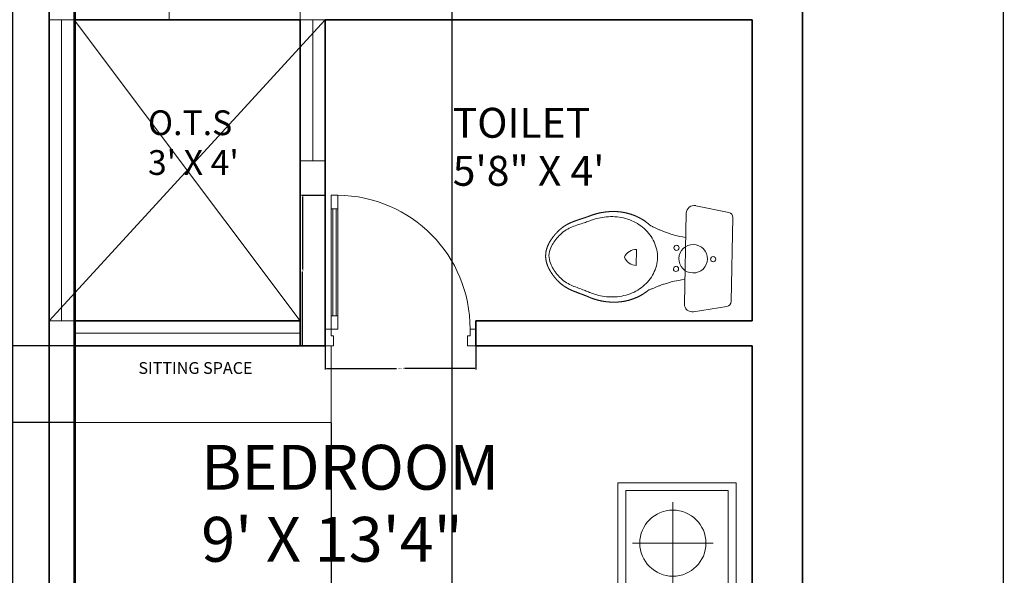
# Model space of a CAD drawing. Units: feet. Extents: x 1993 to 2298, y 2938 to 3641.
# Tile 10 of 11: x 2141 to 2298, y 3468 to 3557. Entities that reach past the tile are written whole.
import ezdxf

# ---------------------------------------------------------------- set-up
doc = ezdxf.new("R2010")
doc.units = ezdxf.units.FT
for name, color, linetype, lineweight in [('A-ANNO-DIMS', 2, 'Continuous', 18), ('A-AREA-IDEN', 7, 'Continuous', 18), ('A-DOOR', 3, 'Continuous', 18), ('A-FLOR-CASE', 8, 'Continuous', 18), ('A-FLOR-FIXT', 9, 'Continuous', 18), ('A-FLOR-OPEN', 8, 'Continuous', 13), ('A-GLAZ', 4, 'Continuous', 13), ('DWV_RED', 7, 'Continuous', 0), ('furniture', 8, 'Continuous', 18), ('WAL', 7, 'Continuous', 35)]:
    doc.layers.add(name, color=color, linetype=linetype, lineweight=lineweight)
doc.styles.add('DIM_FONT', font='SIMPLEX.shx', dxfattribs={"width": 0.8})
doc.styles.get("Standard").update_dxf_attribs({"font": 'arial.ttf'})
doc.dimstyles.get("Standard").update_dxf_attribs({"dimtxt": 0.18, "dimasz": 0.18, "dimexe": 0.18, "dimexo": 0.0625, "dimgap": 0.09, "dimtad": 0, "dimtih": 1, "dimtoh": 1, "dimdec": 4, "dimzin": 0, "dimdsep": 46, "dimtxsty": 'Standard', "dimcen": 0.09, "dimadec": 0, "dimazin": 0, "dimtfac": 1, "dimtdec": 4, "dimtofl": 0, "dimtmove": 0, "dimatfit": 3, "dimfxl": 1, "dimtolj": 1, "dimtzin": 0, "dimarcsym": 0})

# ---------------------------------------------------------------- blocks, each defined once
blk = doc.blocks.new('A$C184E58E8')
for points in [[(825, 900), (825, 820), (865, 820), (865, 900)], [(825, 180), (825, 820), (865, 820), (865, 180)], [(835, 180), (835, 820), (855, 820), (855, 180)], [(825, 100), (825, 180), (865, 180), (865, 100)], [(35, 100), (35, 60), (50, 60), (50, 50), (50, 0), (0, 0), (0, 100)], [(865, 100), (900, 100), (900, 0), (850, 0), (850, 50), (850, 60), (865, 60)]]:
    blk.add_lwpolyline(points, close=True)
blk.add_arc((830, 105), 795, 90.36035, 180.36035)
blk = doc.blocks.new('A$C79766A75')
for p, q in [((0.45, 1.9999), (0, 1.9999)), ((0, 1.9999), (0, 1.5499)), ((0.42, 1.9699), (0.03, 1.9699)), ((0.03, 1.9699), (0.03, 1.5799)), ((0.2304, 1.9125), (0.2304, 1.6061)), ((0.0743, 1.7595), (0.3834, 1.7595)), ((0.03, 1.5799), (0.42, 1.5799)), ((0, 1.5499), (0.45, 1.5499))]:
    blk.add_line(p, q)
blk.add_circle((0.2304, 1.7595), 0.126)
at = {"style": 'DIM_FONT', "text_generation_flag": 4, "width": 0.8, "flags": 9}
for tag in ['XSIZE', 'YSIZE']:
    blk.add_attdef(tag, (1.9506, 2), '', height=0.0005, rotation=180, dxfattribs=at)
blk = doc.blocks.new('A$C6F4D5F33')
at = {"layer": 'DWV_RED'}
for p, q in [((142.3, 403.6), (16.1, 380.5)), ((177.2, 29.5), (177.2, 374.6)), ((0, 42.9), (0, 361.2)), ((376.2, 337), (368.9, 333.5)), ((383.7, 340.2), (376.2, 337)), ((391.3, 343.1), (383.7, 340.2)), ((399.1, 345.6), (391.3, 343.1)), ((407, 347.8), (399.1, 345.6)), ((415, 349.7), (407, 347.8)), ((423.1, 351.2), (415, 349.7)), ((431.3, 352.5), (423.1, 351.2)), ((439.5, 353.3), (431.3, 352.5)), ((447.9, 353.8), (439.5, 353.3)), ((456.2, 354), (447.9, 353.8)), ((464.5, 353.9), (456.2, 354)), ((472.6, 353.4), (464.5, 353.9)), ((480.5, 352.6), (472.6, 353.4)), ((488.1, 351.6), (480.5, 352.6)), ((495.5, 350.4), (488.1, 351.6)), ((502.6, 349.1), (495.5, 350.4)), ((509.4, 347.5), (502.6, 349.1)), ((515.8, 345.9), (509.4, 347.5)), ((521.9, 344.1), (515.8, 345.9)), ((527.5, 342.3), (521.9, 344.1)), ((532.7, 340.4), (527.5, 342.3)), ((537.5, 338.6), (532.7, 340.4)), ((542, 336.9), (537.5, 338.6)), ((546.2, 335.2), (542, 336.9)), ((324, 300.1), (318.7, 294.3)), ((329.7, 305.8), (324, 300.1)), ((335.6, 311.2), (329.7, 305.8)), ((341.8, 316.3), (335.6, 311.2)), ((348.2, 321), (341.8, 316.3)), ((354.9, 325.5), (348.2, 321)), ((361.8, 329.7), (354.9, 325.5)), ((368.9, 333.5), (361.8, 329.7)), ((550.3, 333.5), (546.2, 335.2)), ((554.5, 331.9), (550.3, 333.5)), ((558.9, 330.3), (554.5, 331.9)), ((563.7, 328.6), (558.9, 330.3)), ((568.9, 326.8), (563.7, 328.6)), ((574.3, 324.9), (568.9, 326.8)), ((579.9, 323), (574.3, 324.9)), ((585.7, 321), (579.9, 323)), ((591.4, 318.9), (585.7, 321)), ((597.2, 316.8), (591.4, 318.9)), ((602.9, 314.5), (597.2, 316.8)), ((608.6, 312.1), (602.9, 314.5)), ((614.3, 309.5), (608.6, 312.1)), ((620, 306.6), (614.3, 309.5)), ((625.7, 303.4), (620, 306.6)), ((631.4, 299.9), (625.7, 303.4)), ((637, 296.1), (631.4, 299.9)), ((300.6, 268.4), (296.9, 261.5)), ((304.6, 275.2), (300.6, 268.4)), ((309, 281.8), (304.6, 275.2)), ((313.7, 288.1), (309, 281.8)), ((318.7, 294.3), (313.7, 288.1)), ((642.4, 291.8), (637, 296.1)), ((647.7, 287.3), (642.4, 291.8)), ((652.6, 282.7), (647.7, 287.3)), ((657.3, 277.9), (652.6, 282.7)), ((661.7, 273), (657.3, 277.9)), ((665.8, 268), (661.7, 273)), ((669.7, 263), (665.8, 268)), ((673.4, 258), (669.7, 263)), ((284.8, 224.5), (283.7, 216.9)), ((286.4, 232.1), (284.8, 224.5)), ((288.4, 239.6), (286.4, 232.1)), ((290.8, 247), (288.4, 239.6)), ((293.7, 254.3), (290.8, 247)), ((296.9, 261.5), (293.7, 254.3)), ((362.6, 232.5), (362.6, 171.6)), ((676.8, 253), (673.4, 258)), ((680.1, 247.8), (676.8, 253)), ((683.2, 242.5), (680.1, 247.8)), ((686.1, 236.7), (683.2, 242.5)), ((688.7, 230.6), (686.1, 236.7)), ((691.1, 224), (688.7, 230.6)), ((283.1, 209.2), (282.8, 201.5)), ((282.8, 201.5), (283.1, 193.8)), ((283.7, 216.9), (283.1, 209.2)), ((283.1, 193.8), (283.7, 186.1)), ((692.9, 217), (691.1, 224)), ((694.1, 209.4), (692.9, 217)), ((692.9, 186.1), (694.1, 193.6)), ((694.6, 201.5), (694.1, 209.4)), ((694.1, 193.6), (694.6, 201.5)), ((283.7, 186.1), (284.8, 178.4)), ((284.8, 178.4), (286.4, 170.8)), ((286.4, 170.8), (288.4, 163.3)), ((288.4, 163.3), (290.8, 155.9)), ((290.8, 155.9), (293.7, 148.6)), ((673.4, 145), (676.8, 150.1)), ((676.8, 150.1), (680.1, 155.2)), ((680.1, 155.2), (683.2, 160.6)), ((683.2, 160.6), (686.1, 166.3)), ((686.1, 166.3), (688.7, 172.4)), ((688.7, 172.4), (691.1, 179)), ((691.1, 179), (692.9, 186.1)), ((293.7, 148.6), (296.9, 141.5)), ((296.9, 141.5), (300.6, 134.5)), ((300.6, 134.5), (304.6, 127.7)), ((304.6, 127.7), (309, 121.2)), ((309, 121.2), (313.7, 114.8)), ((313.7, 114.8), (318.7, 108.7)), ((642.4, 111.2), (647.7, 115.7)), ((647.7, 115.7), (652.6, 120.4)), ((652.6, 120.4), (657.3, 125.2)), ((657.3, 125.2), (661.7, 130.1)), ((661.7, 130.1), (665.8, 135)), ((665.8, 135), (669.7, 140)), ((669.7, 140), (673.4, 145)), ((318.7, 108.7), (324, 102.8)), ((324, 102.8), (329.7, 97.2)), ((329.7, 97.2), (335.6, 91.8)), ((335.6, 91.8), (341.8, 86.7)), ((341.8, 86.7), (348.2, 81.9)), ((348.2, 81.9), (354.9, 77.4)), ((354.9, 77.4), (361.8, 73.3)), ((564, 74.5), (569.1, 76.3)), ((569.1, 76.3), (574.6, 78.2)), ((574.6, 78.2), (580.1, 80.1)), ((580.1, 80.1), (585.8, 82.1)), ((585.8, 82.1), (591.5, 84.2)), ((591.5, 84.2), (597.2, 86.3)), ((597.2, 86.3), (602.9, 88.6)), ((602.9, 88.6), (608.6, 91)), ((608.6, 91), (614.3, 93.6)), ((614.3, 93.6), (620, 96.4)), ((620, 96.4), (625.7, 99.6)), ((625.7, 99.6), (631.4, 103.1)), ((631.4, 103.1), (637, 107)), ((637, 107), (642.4, 111.2)), ((361.8, 73.3), (368.9, 69.4)), ((368.9, 69.4), (376.2, 65.9)), ((376.2, 65.9), (383.7, 62.7)), ((383.7, 62.7), (391.3, 59.8)), ((391.3, 59.8), (399.1, 57.3)), ((399.1, 57.3), (407, 55.1)), ((407, 55.1), (415, 53.2)), ((415, 53.2), (423.1, 51.7)), ((423.1, 51.7), (431.3, 50.5)), ((431.3, 50.5), (439.5, 49.6)), ((439.5, 49.6), (447.9, 49.1)), ((447.9, 49.1), (456.2, 48.9)), ((456.2, 48.9), (464.5, 49.1)), ((464.5, 49.1), (472.6, 49.6)), ((472.6, 49.6), (480.5, 50.3)), ((480.5, 50.3), (488.1, 51.3)), ((488.1, 51.3), (495.5, 52.5)), ((495.5, 52.5), (502.7, 53.9)), ((502.7, 53.9), (509.5, 55.4)), ((509.5, 55.4), (515.9, 57.1)), ((515.9, 57.1), (522, 58.9)), ((522, 58.9), (527.7, 60.8)), ((527.7, 60.8), (532.9, 62.6)), ((532.9, 62.6), (537.7, 64.5)), ((537.7, 64.5), (542.3, 66.2)), ((542.3, 66.2), (546.5, 68)), ((546.5, 68), (550.6, 69.6)), ((550.6, 69.6), (554.8, 71.2)), ((554.8, 71.2), (559.2, 72.8)), ((559.2, 72.8), (564, 74.5)), ((142.3, 0.5), (16.1, 23.6))]:
    blk.add_line(p, q, dxfattribs=at)
blk.add_lwpolyline([(177.2, 282.1), (189.7, 283.7), (200.3, 285.4), (209.4, 287.1), (217.2, 288.8), (223.8, 290.5), (229.5, 292.2), (234.5, 293.8), (239, 295.3), (243.3, 296.8), (247.4, 298.1), (251.3, 299.4), (254.9, 300.6), (258.4, 301.7), (261.7, 302.9), (264.8, 304), (267.8, 305.1), (270.6, 306.2), (273.3, 307.3), (275.9, 308.4), (278.5, 309.5), (281.1, 310.7), (283.7, 311.9), (286.3, 313.1), (289.1, 314.3), (291.9, 315.5), (294.8, 316.8), (297.7, 318), (300.5, 319.2), (303.3, 320.3), (305.8, 321.4), (308, 322.3), (310, 323.2), (311.5, 323.8), (312.8, 324.4), (313.8, 324.9), (314.6, 325.3), (315.2, 325.7), (315.7, 326), (316.2, 326.4), (316.7, 326.8), (317.3, 327.3), (318, 327.8), (318.7, 328.4), (319.5, 329), (320.3, 329.7), (321.1, 330.3), (322, 331), (322.9, 331.7), (323.8, 332.4), (324.7, 333.1), (325.6, 333.8), (326.5, 334.4), (327.4, 335.1), (328.3, 335.8), (329.2, 336.4), (330.1, 337.1), (331, 337.7), (331.9, 338.3), (332.9, 339), (333.8, 339.6), (334.7, 340.2), (335.7, 340.8), (336.6, 341.5), (337.6, 342.1), (338.5, 342.7), (339.5, 343.3), (340.4, 343.8), (341.4, 344.4), (342.3, 345), (343.3, 345.6), (344.3, 346.1), (345.2, 346.7), (346.2, 347.3), (347.2, 347.8), (348.2, 348.4), (349.2, 348.9), (350.2, 349.4), (351.1, 349.9), (352.1, 350.5), (353.1, 351), (354.1, 351.5), (355.1, 352), (356.2, 352.5), (357.2, 353), (358.2, 353.5), (359.2, 353.9), (360.2, 354.4), (361.2, 354.9), (362.3, 355.4), (363.3, 355.8), (364.3, 356.3), (365.4, 356.7), (366.4, 357.2), (367.4, 357.6), (368.5, 358), (369.5, 358.4), (370.6, 358.9), (371.6, 359.3), (372.7, 359.7), (373.7, 360.1), (374.8, 360.5), (375.8, 360.9), (376.9, 361.2), (378, 361.6), (379, 362), (380.1, 362.3), (381.2, 362.7), (382.3, 363.1), (383.3, 363.4), (384.4, 363.8), (385.5, 364.1), (386.6, 364.4), (387.7, 364.7), (388.7, 365.1), (389.8, 365.4), (390.9, 365.7), (392, 366), (393.1, 366.3), (394.2, 366.6), (395.3, 366.8), (396.4, 367.1), (397.5, 367.4), (398.6, 367.7), (399.7, 367.9), (400.8, 368.2), (401.9, 368.4), (403, 368.7), (404.1, 368.9), (405.2, 369.1), (406.3, 369.4), (407.4, 369.6), (408.5, 369.8), (409.7, 370), (410.8, 370.2), (411.9, 370.4), (413, 370.6), (414.1, 370.8), (415.3, 371), (416.4, 371.1), (417.5, 371.3), (418.6, 371.5), (419.8, 371.6), (420.9, 371.8), (422, 371.9), (423.1, 372.1), (424.3, 372.2), (425.4, 372.3), (426.5, 372.4), (427.7, 372.6), (428.8, 372.7), (429.9, 372.8), (431.1, 372.9), (432.2, 373), (433.4, 373.1), (434.5, 373.1), (435.6, 373.2), (436.8, 373.3), (437.9, 373.3), (439.1, 373.4), (440.2, 373.5), (441.4, 373.5), (442.5, 373.5), (443.6, 373.6), (444.8, 373.6), (445.9, 373.6), (447.1, 373.6), (448.2, 373.6), (449.3, 373.6), (450.5, 373.6), (451.6, 373.6), (452.8, 373.6), (453.9, 373.6), (455, 373.6), (456.1, 373.5), (457.3, 373.5), (458.4, 373.5), (459.5, 373.4), (460.6, 373.4), (461.7, 373.3), (462.8, 373.2), (463.9, 373.2), (465, 373.1), (466.1, 373), (467.2, 373), (468.3, 372.9), (469.4, 372.8), (470.5, 372.7), (471.5, 372.6), (472.6, 372.5), (473.7, 372.4), (474.7, 372.3), (475.8, 372.1), (476.8, 372), (477.9, 371.9), (478.9, 371.8), (480, 371.6), (481, 371.5), (482, 371.4), (483, 371.2), (484.1, 371.1), (485.1, 370.9), (486.1, 370.8), (487.1, 370.6), (488.1, 370.5), (489.1, 370.3), (490.1, 370.1), (491.1, 370), (492.1, 369.8), (493, 369.6), (494, 369.4), (495, 369.2), (495.9, 369.1), (496.9, 368.9), (497.8, 368.7), (498.8, 368.5), (499.7, 368.3), (500.7, 368.1), (501.6, 367.9), (502.5, 367.7), (503.5, 367.5), (504.4, 367.3), (505.3, 367.1), (506.2, 366.9), (507.1, 366.6), (508, 366.4), (508.9, 366.2), (509.8, 366), (510.7, 365.8), (511.5, 365.5), (512.4, 365.3), (513.3, 365.1), (514.1, 364.8), (515, 364.6), (515.8, 364.4), (516.7, 364.1), (517.5, 363.9), (518.3, 363.6), (519.1, 363.4), (519.9, 363.2), (520.7, 362.9), (521.5, 362.7), (522.3, 362.4), (523.1, 362.2), (523.9, 361.9), (524.6, 361.7), (525.4, 361.4), (526.1, 361.2), (526.9, 360.9), (527.6, 360.7), (528.3, 360.4), (529.1, 360.2), (529.8, 359.9), (530.5, 359.7), (531.2, 359.4), (531.9, 359.2), (532.5, 358.9), (533.2, 358.7), (533.9, 358.4), (534.5, 358.2), (535.2, 358), (535.8, 357.7), (536.4, 357.5), (537.1, 357.2), (537.7, 357), (538.3, 356.8), (538.9, 356.5), (539.5, 356.3), (540.1, 356.1), (540.6, 355.8), (541.2, 355.6), (541.8, 355.4), (542.3, 355.2), (542.9, 355), (543.4, 354.7), (544, 354.5), (544.5, 354.3), (545.1, 354.1), (545.6, 353.9), (546.1, 353.7), (546.6, 353.5), (547.1, 353.3), (547.6, 353.1), (548.2, 352.9), (548.7, 352.7), (549.2, 352.5), (549.6, 352.3), (550.1, 352.1), (550.6, 351.9), (551.1, 351.7), (551.6, 351.5), (552.1, 351.3), (552.6, 351.1), (553.1, 350.9), (553.6, 350.7), (554.1, 350.6), (554.6, 350.4), (555.1, 350.2), (555.6, 350), (556.1, 349.8), (556.7, 349.6), (557.2, 349.4), (557.7, 349.2), (558.3, 349), (558.8, 348.8), (559.4, 348.6), (560, 348.4), (560.5, 348.2), (561.1, 348), (561.7, 347.8), (562.3, 347.6), (562.9, 347.4), (563.5, 347.2), (564.1, 346.9), (564.7, 346.7), (565.4, 346.5), (566, 346.3), (566.6, 346.1), (567.3, 345.8), (567.9, 345.6), (568.6, 345.4), (569.2, 345.2), (569.9, 344.9), (570.6, 344.7), (571.2, 344.5), (571.9, 344.2), (572.6, 344), (573.3, 343.8), (574, 343.5), (574.7, 343.3), (575.4, 343), (576.1, 342.8), (576.8, 342.6), (577.5, 342.3), (578.2, 342.1), (578.9, 341.8), (579.6, 341.6), (580.3, 341.3), (581.1, 341.1), (581.8, 340.8), (582.5, 340.5), (583.3, 340.3), (584, 340), (584.7, 339.8), (585.4, 339.5), (586.2, 339.2), (586.9, 339), (587.7, 338.7), (588.4, 338.4), (589.1, 338.2), (589.9, 337.9), (590.6, 337.6), (591.4, 337.4), (592.1, 337.1), (592.9, 336.8), (593.6, 336.5), (594.4, 336.2), (595.1, 336), (595.9, 335.7), (596.6, 335.4), (597.4, 335.1), (598.2, 334.8), (598.9, 334.5), (599.7, 334.2), (600.4, 333.9), (601.2, 333.6), (602, 333.3), (602.7, 333), (603.5, 332.7), (604.3, 332.4), (605, 332.1), (605.8, 331.7), (606.6, 331.4), (607.3, 331.1), (608.1, 330.7), (608.9, 330.4), (609.7, 330.1), (610.5, 329.7), (611.2, 329.4), (612, 329), (612.8, 328.7), (613.6, 328.3), (614.4, 327.9), (615.2, 327.6), (616, 327.2), (616.8, 326.8), (617.6, 326.4), (618.4, 326), (619.2, 325.6), (620, 325.2), (620.8, 324.8), (621.6, 324.4), (622.4, 324), (623.2, 323.5), (624, 323.1), (624.8, 322.7), (625.6, 322.2), (626.4, 321.8), (627.2, 321.3), (628, 320.8), (628.8, 320.4), (629.6, 319.9), (630.4, 319.4), (631.2, 318.9), (632.1, 318.4), (632.9, 317.9), (633.7, 317.4), (634.5, 316.9), (635.3, 316.3), (636.1, 315.8), (636.9, 315.3), (637.7, 314.7), (638.5, 314.2), (639.3, 313.6), (640.1, 313.1), (640.9, 312.5), (641.7, 311.9), (642.5, 311.3), (643.3, 310.7), (644.1, 310.1), (644.9, 309.5), (645.7, 308.9), (646.4, 308.3), (647.2, 307.7), (648, 307.1), (648.7, 306.4), (649.5, 305.8), (650.3, 305.2), (651, 304.5), (651.8, 303.9), (652.5, 303.3), (653.2, 302.6), (654, 302), (654.7, 301.3), (655.4, 300.6), (656.1, 300), (656.8, 299.3), (657.5, 298.7), (658.2, 298), (658.9, 297.3), (659.6, 296.7), (660.2, 296), (660.9, 295.3), (661.6, 294.7), (662.2, 294), (662.9, 293.3), (663.5, 292.7), (664.2, 292), (664.8, 291.3), (665.4, 290.6), (666, 290), (666.7, 289.3), (667.3, 288.6), (667.9, 287.9), (668.5, 287.2), (669.1, 286.6), (669.7, 285.9), (670.3, 285.2), (670.9, 284.5), (671.4, 283.8), (672, 283.1), (672.6, 282.5), (673.2, 281.8), (673.7, 281.1), (674.3, 280.4), (674.8, 279.7), (675.4, 279), (675.9, 278.3), (676.5, 277.6), (677, 277), (677.5, 276.3), (678.1, 275.6), (678.6, 274.9), (679.1, 274.2), (679.6, 273.5), (680.1, 272.8), (680.6, 272.1), (681.1, 271.4), (681.6, 270.7), (682.1, 270), (682.6, 269.3), (683.1, 268.6), (683.6, 268), (684.1, 267.3), (684.5, 266.6), (685, 265.9), (685.5, 265.2), (686, 264.4), (686.4, 263.7), (686.9, 263), (687.4, 262.3), (687.8, 261.6), (688.3, 260.9), (688.7, 260.1), (689.2, 259.4), (689.6, 258.7), (690.1, 257.9), (690.5, 257.2), (691, 256.4), (691.4, 255.7), (691.9, 254.9), (692.3, 254.1), (692.7, 253.3), (693.2, 252.5), (693.6, 251.7), (694.1, 250.9), (694.5, 250.1), (694.9, 249.3), (695.3, 248.5), (695.8, 247.6), (696.2, 246.8), (696.6, 245.9), (697, 245), (697.4, 244.2), (697.8, 243.3), (698.2, 242.4), (698.6, 241.5), (699, 240.5), (699.4, 239.6), (699.8, 238.7), (700.2, 237.7), (700.6, 236.7), (700.9, 235.8), (701.3, 234.8), (701.6, 233.8), (702, 232.8), (702.3, 231.8), (702.7, 230.7), (703, 229.7), (703.3, 228.6), (703.6, 227.6), (703.9, 226.5), (704.2, 225.4), (704.5, 224.3), (704.7, 223.2), (705, 222.1), (705.2, 220.9), (705.5, 219.8), (705.7, 218.6), (705.9, 217.4), (706.1, 216.3), (706.3, 215.1), (706.4, 213.9), (706.6, 212.7), (706.7, 211.5), (706.9, 210.2), (707, 209), (707.1, 207.8), (707.1, 206.5), (707.2, 205.3), (707.2, 204), (707.3, 202.8), (707.3, 201.5), (707.3, 200.3), (707.2, 199), (707.2, 197.8), (707.1, 196.5), (707.1, 195.3), (707, 194), (706.9, 192.8), (706.7, 191.6), (706.6, 190.4), (706.4, 189.2), (706.3, 188), (706.1, 186.8), (705.9, 185.6), (705.7, 184.4), (705.5, 183.3), (705.2, 182.1), (705, 181), (704.7, 179.9), (704.5, 178.8), (704.2, 177.6), (703.9, 176.6), (703.6, 175.5), (703.3, 174.4), (703, 173.4), (702.7, 172.3), (702.3, 171.3), (702, 170.3), (701.6, 169.3), (701.3, 168.3), (700.9, 167.3), (700.6, 166.3), (700.2, 165.3), (699.8, 164.4), (699.4, 163.4), (699, 162.5), (698.6, 161.6), (698.2, 160.7), (697.8, 159.8), (697.4, 158.9), (697, 158), (696.6, 157.1), (696.2, 156.3), (695.8, 155.4), (695.3, 154.6), (694.9, 153.7), (694.5, 152.9), (694.1, 152.1), (693.6, 151.3), (693.2, 150.5), (692.7, 149.7), (692.3, 148.9), (691.9, 148.1), (691.4, 147.4), (691, 146.6), (690.5, 145.9), (690.1, 145.1), (689.6, 144.4), (689.2, 143.6), (688.7, 142.9), (688.3, 142.2), (687.8, 141.4), (687.4, 140.7), (686.9, 140), (686.4, 139.3), (686, 138.6), (685.5, 137.9), (685, 137.2), (684.5, 136.5), (684.1, 135.8), (683.6, 135.1), (683.1, 134.4), (682.6, 133.7), (682.1, 133), (681.6, 132.3), (681.1, 131.6), (680.6, 130.9), (680.1, 130.2), (679.6, 129.5), (679.1, 128.9), (678.6, 128.2), (678.1, 127.5), (677.5, 126.8), (677, 126.1), (676.5, 125.4), (675.9, 124.7), (675.4, 124), (674.8, 123.3), (674.3, 122.6), (673.7, 122), (673.2, 121.3), (672.6, 120.6), (672, 119.9), (671.4, 119.2), (670.9, 118.5), (670.3, 117.9), (669.7, 117.2), (669.1, 116.5), (668.5, 115.8), (667.9, 115.1), (667.3, 114.4), (666.7, 113.8), (666, 113.1), (665.4, 112.4), (664.8, 111.7), (664.2, 111.1), (663.5, 110.4), (662.9, 109.7), (662.2, 109), (661.6, 108.4), (660.9, 107.7), (660.2, 107), (659.6, 106.4), (658.9, 105.7), (658.2, 105), (657.5, 104.4), (656.8, 103.7), (656.1, 103.1), (655.4, 102.4), (654.7, 101.7), (654, 101.1), (653.2, 100.4), (652.5, 99.8), (651.8, 99.1), (651, 98.5), (650.3, 97.9), (649.5, 97.2), (648.7, 96.6), (648, 96), (647.2, 95.3), (646.4, 94.7), (645.7, 94.1), (644.9, 93.5), (644.1, 92.9), (643.3, 92.3), (642.5, 91.7), (641.7, 91.1), (640.9, 90.6), (640.1, 90), (639.3, 89.4), (638.5, 88.9), (637.7, 88.3), (636.9, 87.8), (636.1, 87.2), (635.3, 86.7), (634.5, 86.2), (633.7, 85.7), (632.9, 85.1), (632.1, 84.6), (631.3, 84.1), (630.4, 83.7), (629.6, 83.2), (628.8, 82.7), (628, 82.2), (627.2, 81.8), (626.4, 81.3), (625.6, 80.8), (624.8, 80.4), (624, 80), (623.2, 79.5), (622.4, 79.1), (621.6, 78.7), (620.8, 78.3), (620, 77.8), (619.2, 77.4), (618.4, 77), (617.6, 76.7), (616.8, 76.3), (616, 75.9), (615.2, 75.5), (614.4, 75.1), (613.6, 74.8), (612.8, 74.4), (612.1, 74), (611.3, 73.7), (610.5, 73.3), (609.7, 73), (608.9, 72.7), (608.2, 72.3), (607.4, 72), (606.6, 71.7), (605.8, 71.3), (605.1, 71), (604.3, 70.7), (603.5, 70.4), (602.8, 70.1), (602, 69.8), (601.3, 69.5), (600.5, 69.1), (599.7, 68.9), (599, 68.6), (598.2, 68.3), (597.5, 68), (596.7, 67.7), (596, 67.4), (595.2, 67.1), (594.5, 66.8), (593.7, 66.5), (593, 66.3), (592.2, 66), (591.5, 65.7), (590.7, 65.4), (590, 65.2), (589.3, 64.9), (588.5, 64.6), (587.8, 64.4), (587, 64.1), (586.3, 63.8), (585.6, 63.6), (584.8, 63.3), (584.1, 63.1), (583.4, 62.8), (582.7, 62.5), (581.9, 62.3), (581.2, 62), (580.5, 61.8), (579.8, 61.5), (579.1, 61.3), (578.4, 61), (577.7, 60.8), (577, 60.6), (576.3, 60.3), (575.6, 60.1), (574.9, 59.8), (574.2, 59.6), (573.5, 59.4), (572.8, 59.1), (572.1, 58.9), (571.5, 58.7), (570.8, 58.4), (570.1, 58.2), (569.5, 58), (568.8, 57.7), (568.2, 57.5), (567.5, 57.3), (566.9, 57.1), (566.2, 56.8), (565.6, 56.6), (565, 56.4), (564.4, 56.2), (563.8, 56), (563.2, 55.8), (562.6, 55.5), (562, 55.3), (561.4, 55.1), (560.8, 54.9), (560.2, 54.7), (559.7, 54.5), (559.1, 54.3), (558.6, 54.1), (558, 53.9), (557.5, 53.7), (557, 53.5), (556.5, 53.3), (555.9, 53.1), (555.4, 53), (554.9, 52.8), (554.4, 52.6), (553.9, 52.4), (553.4, 52.2), (552.9, 52), (552.4, 51.8), (551.9, 51.6), (551.5, 51.4), (551, 51.2), (550.5, 51.1), (550, 50.9), (549.5, 50.7), (549, 50.5), (548.5, 50.3), (548, 50.1), (547.5, 49.9), (546.9, 49.7), (546.4, 49.4), (545.9, 49.2), (545.4, 49), (544.8, 48.8), (544.3, 48.6), (543.8, 48.4), (543.2, 48.2), (542.6, 47.9), (542.1, 47.7), (541.5, 47.5), (540.9, 47.3), (540.4, 47), (539.8, 46.8), (539.2, 46.6), (538.6, 46.3), (538, 46.1), (537.3, 45.9), (536.7, 45.6), (536.1, 45.4), (535.4, 45.1), (534.8, 44.9), (534.1, 44.6), (533.5, 44.4), (532.8, 44.1), (532.1, 43.9), (531.4, 43.6), (530.7, 43.4), (530, 43.1), (529.3, 42.9), (528.6, 42.6), (527.8, 42.4), (527.1, 42.1), (526.4, 41.9), (525.6, 41.6), (524.8, 41.4), (524.1, 41.1), (523.3, 40.9), (522.5, 40.6), (521.7, 40.4), (520.9, 40.1), (520.1, 39.9), (519.3, 39.6), (518.5, 39.4), (517.7, 39.1), (516.8, 38.9), (516, 38.6), (515.1, 38.4), (514.3, 38.2), (513.4, 37.9), (512.5, 37.7), (511.7, 37.5), (510.8, 37.2), (509.9, 37), (509, 36.8), (508.1, 36.6), (507.2, 36.3), (506.3, 36.1), (505.4, 35.9), (504.5, 35.7), (503.6, 35.5), (502.6, 35.3), (501.7, 35.1), (500.8, 34.9), (499.8, 34.7), (498.9, 34.5), (497.9, 34.3), (497, 34.1), (496, 33.9), (495, 33.7), (494.1, 33.5), (493.1, 33.4), (492.1, 33.2), (491.1, 33), (490.1, 32.8), (489.1, 32.7), (488.1, 32.5), (487.1, 32.3), (486.1, 32.2), (485.1, 32), (484.1, 31.9), (483.1, 31.7), (482.1, 31.6), (481, 31.4), (480, 31.3), (478.9, 31.2), (477.9, 31.1), (476.9, 30.9), (475.8, 30.8), (474.7, 30.7), (473.7, 30.6), (472.6, 30.5), (471.6, 30.4), (470.5, 30.3), (469.4, 30.2), (468.3, 30.1), (467.2, 30), (466.1, 29.9), (465, 29.8), (463.9, 29.8), (462.8, 29.7), (461.7, 29.6), (460.6, 29.6), (459.5, 29.5), (458.4, 29.5), (457.3, 29.4), (456.1, 29.4), (455, 29.4), (453.9, 29.3), (452.8, 29.3), (451.6, 29.3), (450.5, 29.3), (449.3, 29.3), (448.2, 29.3), (447.1, 29.3), (445.9, 29.3), (444.8, 29.3), (443.6, 29.4), (442.5, 29.4), (441.4, 29.4), (440.2, 29.5), (439.1, 29.5), (437.9, 29.6), (436.8, 29.7), (435.6, 29.7), (434.5, 29.8), (433.4, 29.9), (432.2, 30), (431.1, 30.1), (429.9, 30.2), (428.8, 30.3), (427.7, 30.4), (426.5, 30.5), (425.4, 30.6), (424.3, 30.7), (423.1, 30.9), (422, 31), (420.9, 31.2), (419.8, 31.3), (418.6, 31.5), (417.5, 31.6), (416.4, 31.8), (415.3, 32), (414.1, 32.2), (413, 32.3), (411.9, 32.5), (410.8, 32.7), (409.7, 32.9), (408.5, 33.1), (407.4, 33.4), (406.3, 33.6), (405.2, 33.8), (404.1, 34), (403, 34.3), (401.9, 34.5), (400.8, 34.8), (399.7, 35), (398.6, 35.3), (397.5, 35.5), (396.4, 35.8), (395.3, 36.1), (394.2, 36.4), (393.1, 36.7), (392, 37), (390.9, 37.3), (389.8, 37.6), (388.7, 37.9), (387.7, 38.2), (386.6, 38.5), (385.5, 38.9), (384.4, 39.2), (383.3, 39.5), (382.3, 39.9), (381.2, 40.2), (380.1, 40.6), (379, 41), (378, 41.3), (376.9, 41.7), (375.8, 42.1), (374.8, 42.5), (373.7, 42.9), (372.7, 43.3), (371.6, 43.7), (370.6, 44.1), (369.5, 44.5), (368.5, 44.9), (367.4, 45.4), (366.4, 45.8), (365.4, 46.2), (364.3, 46.7), (363.3, 47.1), (362.3, 47.6), (361.2, 48), (360.2, 48.5), (359.2, 49), (358.2, 49.5), (357.2, 50), (356.2, 50.5), (355.1, 50.9), (354.1, 51.5), (353.1, 52), (352.1, 52.5), (351.1, 53), (350.2, 53.5), (349.2, 54.1), (348.2, 54.6), (347.2, 55.1), (346.2, 55.7), (345.2, 56.2), (344.3, 56.8), (343.3, 57.4), (342.3, 57.9), (341.4, 58.5), (340.4, 59.1), (339.5, 59.7), (338.5, 60.3), (337.6, 60.9), (336.6, 61.5), (335.7, 62.1), (334.7, 62.7), (333.8, 63.3), (332.9, 64), (331.9, 64.6), (331, 65.2), (330.1, 65.9), (329.2, 66.5), (328.3, 67.2), (327.4, 67.8), (326.5, 68.5), (325.6, 69.2), (324.7, 69.9), (323.8, 70.5), (322.9, 71.2), (322, 71.9), (321.1, 72.6), (320.3, 73.3), (319.5, 74), (318.7, 74.6), (317.9, 75.3), (317.2, 75.9), (316.5, 76.4), (315.9, 76.9), (315.3, 77.4), (314.6, 77.9), (313.9, 78.5), (313, 79), (311.9, 79.6), (310.6, 80.3), (309, 81.1), (307.1, 82), (304.9, 82.9), (302.5, 84), (299.9, 85.1), (297.2, 86.3), (294.4, 87.5), (291.6, 88.7), (288.8, 89.9), (286.2, 91.1), (283.6, 92.3), (281, 93.4), (278.5, 94.6), (275.9, 95.7), (273.3, 96.8), (270.6, 97.9), (267.8, 99), (264.8, 100.1), (261.7, 101.2), (258.4, 102.4), (254.9, 103.5), (251.3, 104.7), (247.4, 106), (243.3, 107.3), (239, 108.8), (234.5, 110.3), (229.5, 111.9), (223.8, 113.6), (217.2, 115.3), (209.4, 117), (200.3, 118.7), (189.7, 120.4), (177.2, 122)], dxfattribs=at)
for centre, major_axis, start_param, end_param in [((19.7, 361.2), (-13.9, 13.9), 5.678651, 7.068583), ((147.6, 374.6), (-20.9, 20.9), 3.926991, 5.678651), ((147.6, 202.1), (-38.3, 38.3), 0.785398, 7.068583), ((211.6, 242.1), (-6.96, 6.96), 0.785398, 7.068583), ((362.6, 182.9), (-35.1, -35.1), 2.753037, 3.926991), ((71.5, 202.2), (-6.96, -6.96), -0.785398, 5.497787), ((362.6, 221.2), (-35.1, 35.1), 2.356194, 3.530149), ((211.6, 162), (-6.96, 6.96), 0.785398, 7.068583), ((19.7, 42.9), (-13.9, -13.9), -0.785398, 0.604534), ((147.6, 29.5), (-20.9, -20.9), 0.604534, 2.356194)]:
    blk.add_ellipse(centre, major_axis=major_axis, ratio=1, start_param=start_param, end_param=end_param, dxfattribs=at)
blk = doc.blocks.new('*D24')
at = {"layer": 'A-ANNO-DIMS', "color": 0, "lineweight": -2, "transparency": 16777216}
for p, q in [((2189.76, 3504.47), (2189.76, 3500.75)), ((2213.76, 3504.47), (2213.76, 3500.75)), ((2189.94, 3500.93), (2201.13, 3500.93)), ((2213.58, 3500.93), (2202.38, 3500.93))]:
    blk.add_line(p, q, dxfattribs=at)
at = {"layer": 'A-ANNO-DIMS', "color": 0, "transparency": 16777216}
for points in [[(2189.94, 3500.96), (2189.94, 3500.9), (2189.76, 3500.93)], [(2213.58, 3500.96), (2213.58, 3500.9), (2213.76, 3500.93)]]:
    blk.add_solid(points, dxfattribs=at)
at = {"layer": 'Defpoints', "color": 0, "transparency": 16777216}
for p in [(2189.76, 3504.53), (2213.76, 3504.53), (2189.76, 3500.93)]:
    blk.add_point(p, dxfattribs=at)
at = {"layer": 'A-ANNO-DIMS', "color": 0, "transparency": 16777216, "insert": (2201.76, 3500.93), "char_height": 0.18, "attachment_point": 5}
blk.add_mtext('\\A1;DOOR 24', dxfattribs=at)
blk = doc.blocks.new('*D25')
at = {"layer": 'A-ANNO-DIMS', "color": 0, "lineweight": -2, "transparency": 16777216}
for p, q in [((2189.7, 3528.53), (2185.98, 3528.53)), ((2186.16, 3528.35), (2186.16, 3516.71)), ((2186.16, 3504.71), (2186.16, 3516.35)), ((2189.7, 3504.53), (2185.98, 3504.53))]:
    blk.add_line(p, q, dxfattribs=at)
at = {"layer": 'A-ANNO-DIMS', "color": 0, "transparency": 16777216}
for points in [[(2186.13, 3528.35), (2186.19, 3528.35), (2186.16, 3528.53)], [(2186.13, 3504.71), (2186.19, 3504.71), (2186.16, 3504.53)]]:
    blk.add_solid(points, dxfattribs=at)
at = {"layer": 'Defpoints', "color": 0, "transparency": 16777216}
for p in [(2186.16, 3528.53), (2189.76, 3528.53), (2189.76, 3504.53)]:
    blk.add_point(p, dxfattribs=at)
at = {"layer": 'A-ANNO-DIMS', "color": 0, "transparency": 16777216, "insert": (2186.16, 3516.53), "char_height": 0.18, "attachment_point": 5}
blk.add_mtext('\\A1;24', dxfattribs=at)
blk = doc.blocks.new('*D55')
at = {"layer": 'A-ANNO-DIMS', "color": 0, "lineweight": -2, "transparency": 16777216}
for p, q in [((2265.82, 3608.53), (2297.9, 3608.53)), ((2297.72, 3608.35), (2297.72, 3308.72)), ((2297.72, 3008.71), (2297.72, 3308.35)), ((2265.82, 3008.53), (2297.9, 3008.53))]:
    blk.add_line(p, q, dxfattribs=at)
at = {"layer": 'A-ANNO-DIMS', "color": 0, "transparency": 16777216}
for points in [[(2297.69, 3608.35), (2297.75, 3608.35), (2297.72, 3608.53)], [(2297.69, 3008.71), (2297.75, 3008.71), (2297.72, 3008.53)]]:
    blk.add_solid(points, dxfattribs=at)
at = {"layer": 'Defpoints', "color": 0, "transparency": 16777216}
for p in [(2265.76, 3608.53), (2297.72, 3608.53), (2265.76, 3008.53)]:
    blk.add_point(p, dxfattribs=at)
at = {"layer": 'A-ANNO-DIMS', "color": 0, "transparency": 16777216, "insert": (2297.72, 3308.53), "char_height": 0.18, "attachment_point": 5}
blk.add_mtext('\\A1;600', dxfattribs=at)
blk = doc.blocks.new('*D59')
at = {"layer": 'A-ANNO-DIMS', "color": 0, "lineweight": -2, "transparency": 16777216}
for p, q in [((2140, 3048.6), (2140, 3640.68)), ((2140.18, 3640.5), (2144.79, 3640.5)), ((2149.82, 3640.5), (2145.21, 3640.5)), ((2150, 3048.6), (2150, 3640.68))]:
    blk.add_line(p, q, dxfattribs=at)
at = {"layer": 'A-ANNO-DIMS', "color": 0, "transparency": 16777216}
for points in [[(2140.18, 3640.53), (2140.18, 3640.47), (2140, 3640.5)], [(2149.82, 3640.53), (2149.82, 3640.47), (2150, 3640.5)]]:
    blk.add_solid(points, dxfattribs=at)
at = {"layer": 'Defpoints', "color": 0, "transparency": 16777216}
for p in [(2150, 3640.5), (2140, 3048.53), (2150, 3048.53)]:
    blk.add_point(p, dxfattribs=at)
at = {"layer": 'A-ANNO-DIMS', "color": 0, "transparency": 16777216, "insert": (2145, 3640.5), "char_height": 0.18, "attachment_point": 5}
blk.add_mtext('\\A1;10', dxfattribs=at)
blk = doc.blocks.new('*D69')
at = {"layer": 'A-ANNO-DIMS', "color": 0, "lineweight": -2, "transparency": 16777216}
for p, q in [((2149.76, 3492.27), (2149.76, 2937.86)), ((2190.69, 3492.27), (2190.69, 2937.86)), ((2149.94, 2938.03), (2169.83, 2938.03)), ((2190.51, 2938.03), (2170.62, 2938.03))]:
    blk.add_line(p, q, dxfattribs=at)
at = {"layer": 'A-ANNO-DIMS', "color": 0, "transparency": 16777216}
for points in [[(2149.94, 2938.07), (2149.94, 2938.01), (2149.76, 2938.03)], [(2190.51, 2938.07), (2190.51, 2938.01), (2190.69, 2938.03)]]:
    blk.add_solid(points, dxfattribs=at)
at = {"layer": 'Defpoints', "color": 0, "transparency": 16777216}
for p in [(2149.76, 3492.33), (2190.69, 3492.33), (2190.69, 2938.03)]:
    blk.add_point(p, dxfattribs=at)
at = {"layer": 'A-ANNO-DIMS', "color": 0, "transparency": 16777216, "insert": (2170.23, 2938.03), "char_height": 0.18, "attachment_point": 5}
blk.add_mtext('\\A1;40.93', dxfattribs=at)
blk = doc.blocks.new('*D70')
at = {"layer": 'A-ANNO-DIMS', "color": 0, "lineweight": -2, "transparency": 16777216}
for p, q in [((2149.7, 3504.53), (1993.61, 3504.53)), ((1993.79, 3504.35), (1993.79, 3498.61)), ((1993.79, 3492.51), (1993.79, 3498.25)), ((2149.7, 3492.33), (1993.61, 3492.33))]:
    blk.add_line(p, q, dxfattribs=at)
at = {"layer": 'A-ANNO-DIMS', "color": 0, "transparency": 16777216}
for points in [[(1993.76, 3504.35), (1993.82, 3504.35), (1993.79, 3504.53)], [(1993.76, 3492.51), (1993.82, 3492.51), (1993.79, 3492.33)]]:
    blk.add_solid(points, dxfattribs=at)
at = {"layer": 'Defpoints', "color": 0, "transparency": 16777216}
for p in [(1993.79, 3504.53), (2149.76, 3504.53), (2149.76, 3492.33)]:
    blk.add_point(p, dxfattribs=at)
at = {"layer": 'A-ANNO-DIMS', "color": 0, "transparency": 16777216, "insert": (1993.79, 3498.43), "char_height": 0.18, "attachment_point": 5}
blk.add_mtext('\\A1;12.2', dxfattribs=at)
blk = doc.blocks.new('*D73')
at = {"layer": 'A-ANNO-DIMS', "color": 0, "lineweight": -2, "transparency": 16777216}
for p, q in [((2149.76, 3105.6), (2149.76, 3640.68)), ((2149.94, 3640.5), (2179.49, 3640.5)), ((2209.82, 3640.5), (2180.27, 3640.5)), ((2210, 3105.6), (2210, 3640.68))]:
    blk.add_line(p, q, dxfattribs=at)
at = {"layer": 'A-ANNO-DIMS', "color": 0, "transparency": 16777216}
for points in [[(2149.94, 3640.53), (2149.94, 3640.47), (2149.76, 3640.5)], [(2209.82, 3640.53), (2209.82, 3640.47), (2210, 3640.5)]]:
    blk.add_solid(points, dxfattribs=at)
at = {"layer": 'Defpoints', "color": 0, "transparency": 16777216}
for p in [(2210, 3640.5), (2149.76, 3105.53), (2210, 3105.53)]:
    blk.add_point(p, dxfattribs=at)
at = {"layer": 'A-ANNO-DIMS', "color": 0, "transparency": 16777216, "insert": (2179.88, 3640.5), "char_height": 0.18, "attachment_point": 5}
blk.add_mtext('\\A1;60.24', dxfattribs=at)

msp = doc.modelspace()

# ---------------------------------------------------------------- linework, layer by layer
at = {"layer": 'A-FLOR-CASE'}
for p, q in [((2190.6917, 3507.2005), (2190.6917, 3506.1338)), ((2190.6917, 3504.5338), (2190.6917, 3492.3338)), ((2190.6917, 3492.3338), (2149.7583, 3492.3338))]:
    msp.add_line(p, q, dxfattribs=at)
at = {"layer": 'A-FLOR-OPEN'}
for p, q in [((2189.7583, 3556.5338), (2145.7583, 3508.5338)), ((2149.7583, 3556.5338), (2185.7583, 3508.5338))]:
    msp.add_line(p, q, dxfattribs=at)
at = {"layer": 'A-GLAZ'}
for p, q in [((2164.9041, 3560.5338), (2164.9041, 3556.5338)), ((2185.7583, 3556.5338), (2185.7583, 3560.5338)), ((2149.7583, 3556.5338), (2145.7583, 3556.5338)), ((2147.7583, 3508.5338), (2147.7583, 3556.5338)), ((2185.7583, 3556.5338), (2189.7583, 3556.5338)), ((2187.7583, 3534.0155), (2187.7583, 3556.5338)), ((2185.7583, 3534.0155), (2189.7583, 3534.0155)), ((2149.7583, 3508.5338), (2145.7583, 3508.5338)), ((2149.7583, 3508.5338), (2149.7583, 3504.5338)), ((2149.7583, 3506.5338), (2185.7583, 3506.5338))]:
    msp.add_line(p, q, dxfattribs=at)
at = {"layer": 'WAL'}
for p, q in [((2265.7583, 3608.5338), (2265.7583, 3008.5338)), ((2145.7583, 3432.5338), (2145.7583, 3560.5338)), ((2149.7583, 3556.5338), (2185.7583, 3556.5338)), ((2149.7583, 3508.5338), (2149.7583, 3556.5338)), ((2185.7583, 3504.5338), (2185.7583, 3556.5338)), ((2189.7583, 3504.5338), (2189.7583, 3556.5338)), ((2189.7583, 3556.5338), (2257.7583, 3556.5338)), ((2257.7583, 3556.5338), (2257.7583, 3508.5338)), ((2149.7583, 3508.5338), (2185.7583, 3508.5338)), ((2213.7583, 3504.5338), (2213.7583, 3508.5338)), ((2213.7583, 3508.5338), (2257.7583, 3508.5338)), ((2149.7583, 3504.5338), (2189.7583, 3504.5338)), ((2149.7583, 3380.5338), (2149.7583, 3504.5338)), ((2213.7583, 3504.5338), (2257.7583, 3504.5338)), ((2257.7583, 3504.5338), (2257.7583, 3344.5338))]:
    msp.add_line(p, q, dxfattribs=at)

# ---------------------------------------------------------------- block references
at = {"layer": 'A-DOOR', "xscale": -0.0266666666666671, "yscale": 0.0266666666666671, "zscale": 0.0266666666666671}
msp.add_blockref('A$C184E58E8', (2213.7583, 3504.5338), dxfattribs=at)
at = {"layer": 'A-FLOR-FIXT', "xscale": 0.0419889779106581, "yscale": 0.0419889779106581, "zscale": 0.0419889779106581, "rotation": 178.7655746873133}
msp.add_blockref('A$C6F4D5F33', (2254.7389, 3526.7761), dxfattribs=at)
at = {"layer": 'furniture', "xscale": 41.83725109546206, "yscale": 41.83725109546206, "zscale": 41.83725109546206, "rotation": 270}
msp.add_blockref('A$C79766A75', (2171.5191, 3482.724), dxfattribs=at)

# ---------------------------------------------------------------- texts
at = {"layer": 'A-AREA-IDEN'}
for s, height, p in [('O.T.S', 3.94616, (2161.5219, 3538.1285)), ('TOILET', 4.76705, (2210.0734, 3537.7118)), ("3' X 4'", 3.94616, (2161.5219, 3531.7893)), ('5\'8" X 4\'', 4.76705, (2210.0734, 3530.054)), ('SITTING SPACE', 1.880693, (2160, 3500.067)), ('BEDROOM', 7.14808, (2170, 3481.6047)), ('9\' X 13\'4"', 7.14808, (2170, 3470.1219))]:
    msp.add_text(s, height=height, dxfattribs=at).set_placement(p)

# ---------------------------------------------------------------- dimensions: what is measured, and where the dimension line sits
at = {"layer": 'A-ANNO-DIMS'}
for base, p1, p2, override, picture, middle in [((2150, 3640.4988), (2140, 3048.5338), (2150, 3048.5338), {"dimdec": 0, "dimlfac": 1, "dimrnd": 0, "dimzin": 0, "dimdsep": 46, "dimlunit": 2}, '*D59', (2145, 3640.4988)), ((2210, 3640.4988), (2149.7583, 3105.5338), (2210, 3105.5338), {"dimdec": 2, "dimlfac": 1, "dimrnd": 0, "dimzin": 0, "dimdsep": 46, "dimlunit": 2}, '*D73', (2179.8792, 3640.4988)), ((2190.6917, 2938.035), (2149.7583, 3492.3338), (2190.6917, 3492.3338), {"dimdec": 2, "dimlfac": 1, "dimrnd": 0, "dimzin": 0, "dimdsep": 46, "dimlunit": 2}, '*D69', (2170.225, 2938.035))]:
    dim = msp.add_linear_dim(base=base, p1=p1, p2=p2, dimstyle='Standard', override=override, dxfattribs=at)
    dim.commit()
    dim.dimension.update_dxf_attribs({"geometry": picture, "text_midpoint": middle})
for base, p1, p2, override, picture, middle in [((2297.7233, 3608.5338), (2265.7583, 3008.5338), (2265.7583, 3608.5338), {"dimdec": 0, "dimlfac": 1, "dimrnd": 0, "dimzin": 0, "dimdsep": 46, "dimlunit": 2}, '*D55', (2297.7233, 3308.5338)), ((2186.1583, 3528.5338), (2189.7583, 3504.5338), (2189.7583, 3528.5338), {"dimdec": 0, "dimlfac": 1, "dimrnd": 0, "dimzin": 0, "dimdsep": 46, "dimlunit": 2}, '*D25', (2186.1583, 3516.5338)), ((1993.7933, 3504.5338), (2149.7583, 3492.3338), (2149.7583, 3504.5338), {"dimdec": 1, "dimlfac": 1, "dimrnd": 0, "dimzin": 0, "dimdsep": 46, "dimlunit": 2}, '*D70', (1993.7933, 3498.4338))]:
    dim = msp.add_linear_dim(base=base, p1=p1, p2=p2, angle=90, dimstyle='Standard', override=override, dxfattribs=at)
    dim.commit()
    dim.dimension.update_dxf_attribs({"geometry": picture, "text_midpoint": middle})
dim = msp.add_linear_dim(base=(2189.7583, 3500.9338), p1=(2213.7583, 3504.5338), p2=(2189.7583, 3504.5338), angle=180, text='DOOR <>', dimstyle='Standard', override={"dimdec": 0, "dimlfac": 1, "dimrnd": 0, "dimzin": 0, "dimdsep": 46, "dimlunit": 2}, dxfattribs=at)
dim.commit()
dim.dimension.update_dxf_attribs({"geometry": '*D24', "text_midpoint": (2201.7583, 3500.9338)})

doc.saveas('drawing.dxf')
